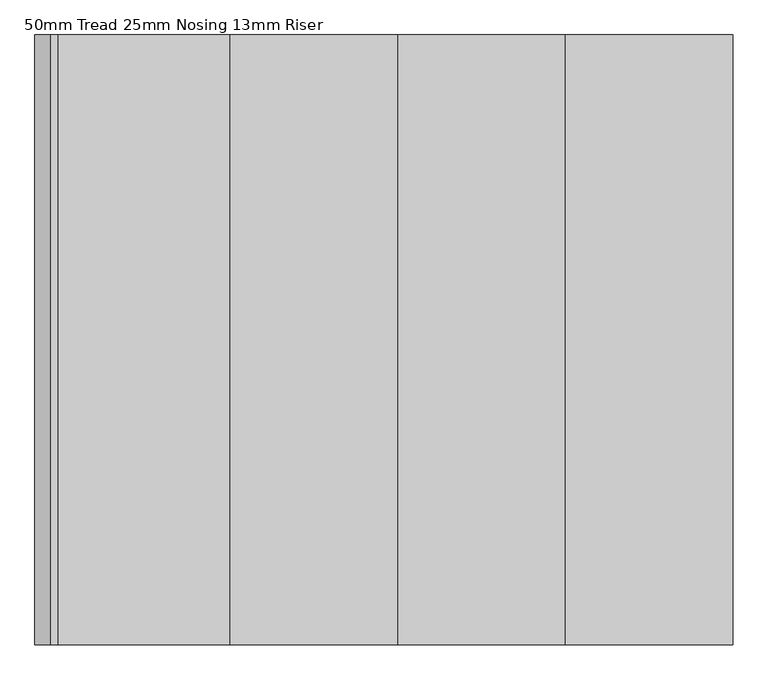
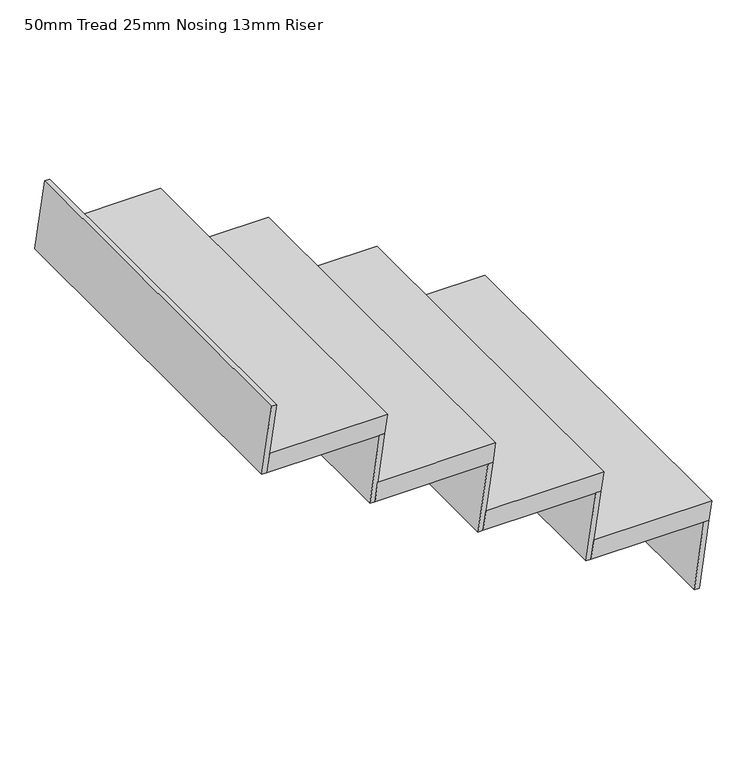
"""IFC4 building model written with IfcOpenShell, lengths in millimetres: stair flight geometry, 50mm Tread 25mm Nosing 13mm Riser."""

from ifc_helpers import new_model, si_unit, frame, origin, place, context, project, spatial, polyline, outline, extrude, source, transform, mapped, element, save


def stair_flight_50mm_tread_25mm_nosing_13mm_riser_dbe7f446(model_context):
    return source(origin(), model_context, "Body", "SweptSolid", [
        extrude(outline(polyline([(1391.3043478, -7089.5726707), (1391.3043478, -7389.5726707), (1341.3043478, -7396.7601707), (1341.3043478, -7096.7601707), (1391.3043478, -7089.5726707)])), frame((0.0, -1069.1062768, 0.0), z_axis=(0.0, 1.0, 0.0), x_axis=(0.0, 0.0, 1.0)), (0.0, 0.0, 1.0), 1000.0257813),
        extrude(outline(polyline([(1341.3043478, -7096.7601707), (1341.3043478, -7109.3886607), (1167.3913043, -7134.3886607), (1167.3913043, -7121.7601707), (1341.3043478, -7096.7601707)])), frame((0.0, -1069.1062768, 0.0), z_axis=(0.0, 1.0, 0.0), x_axis=(0.0, 0.0, 1.0)), (0.0, 0.0, 1.0), 1000.0257812),
        extrude(outline(polyline([(1515.2173913, -7371.7601707), (1515.2173913, -7384.3886607), (1341.3043478, -7409.3886607), (1341.3043478, -7396.7601707), (1515.2173913, -7371.7601707)])), frame((0.0, -1069.1062768, 0.0), z_axis=(0.0, 1.0, 0.0), x_axis=(0.0, 0.0, 1.0)), (0.0, 0.0, 1.0), 1000.0257812),
        extrude(outline(polyline([(1565.2173913, -7364.5726707), (1565.2173913, -7664.5726707), (1515.2173913, -7671.7601707), (1515.2173913, -7371.7601707), (1565.2173913, -7364.5726707)])), frame((0.0, -1069.1062768, 0.0), z_axis=(0.0, 1.0, 0.0), x_axis=(0.0, 0.0, 1.0)), (0.0, 0.0, 1.0), 1000.0257813),
        extrude(outline(polyline([(1689.1304348, -7646.7601707), (1689.1304348, -7659.3886607), (1515.2173913, -7684.3886607), (1515.2173913, -7671.7601707), (1689.1304348, -7646.7601707)])), frame((0.0, -1069.1062768, 0.0), z_axis=(0.0, 1.0, 0.0), x_axis=(0.0, 0.0, 1.0)), (0.0, 0.0, 1.0), 1000.0257813),
        extrude(outline(polyline([(1739.1304348, -7639.5726707), (1739.1304348, -7939.5726707), (1689.1304348, -7946.7601707), (1689.1304348, -7646.7601707), (1739.1304348, -7639.5726707)])), frame((0.0, -1069.1062768, 0.0), z_axis=(0.0, 1.0, 0.0), x_axis=(0.0, 0.0, 1.0)), (0.0, 0.0, 1.0), 1000.0257813),
        extrude(outline(polyline([(1863.0434783, -7921.7601707), (1863.0434783, -7934.3886607), (1689.1304348, -7959.3886607), (1689.1304348, -7946.7601707), (1863.0434783, -7921.7601707)])), frame((0.0, -1069.1062768, 0.0), z_axis=(0.0, 1.0, 0.0), x_axis=(0.0, 0.0, 1.0)), (0.0, 0.0, 1.0), 1000.0257813),
        extrude(outline(polyline([(2036.9565217, -8196.7601707), (2036.9565217, -8209.3886607), (1863.0434783, -8234.3886607), (1863.0434783, -8221.7601707), (2036.9565217, -8196.7601707)])), frame((0.0, -1069.1062768, 0.0), z_axis=(0.0, 1.0, 0.0), x_axis=(0.0, 0.0, 1.0)), (0.0, 0.0, 1.0), 1000.0257812),
        extrude(outline(polyline([(1913.0434783, -7914.5726707), (1913.0434783, -8214.5726707), (1863.0434783, -8221.7601707), (1863.0434783, -7921.7601707), (1913.0434783, -7914.5726707)])), frame((0.0, -1069.1062768, 0.0), z_axis=(0.0, 1.0, 0.0), x_axis=(0.0, 0.0, 1.0)), (0.0, 0.0, 1.0), 1000.0257813),
    ])


if __name__ == "__main__":
    model = new_model("IFC4")
    model_context = context("Model", 3, world=origin())
    ifc_project = project(units=[si_unit("LENGTHUNIT", "METRE", prefix="MILLI")], contexts=[model_context])
    site = spatial("IfcSite", under=ifc_project)
    building = spatial("IfcBuilding", under=site)
    placement = place(None, origin())
    stair_flight_50mm_tread_25mm_nosing_13mm_riser_shape = stair_flight_50mm_tread_25mm_nosing_13mm_riser_dbe7f446(model_context)
    element("IfcStairFlight", 1, ObjectType="50mm Tread 25mm Nosing 13mm Riser", at=placement, inside=building, context=model_context, shape_type="MappedRepresentation", body=[
        mapped(stair_flight_50mm_tread_25mm_nosing_13mm_riser_shape, transform((0.0, 0.0, 0.0), x_axis=(1.0, 0.0, 0.0), y_axis=(0.0, 1.0, 0.0), z_axis=(0.0, 0.0, 1.0))),
    ])
    save(model, "model.ifc")
